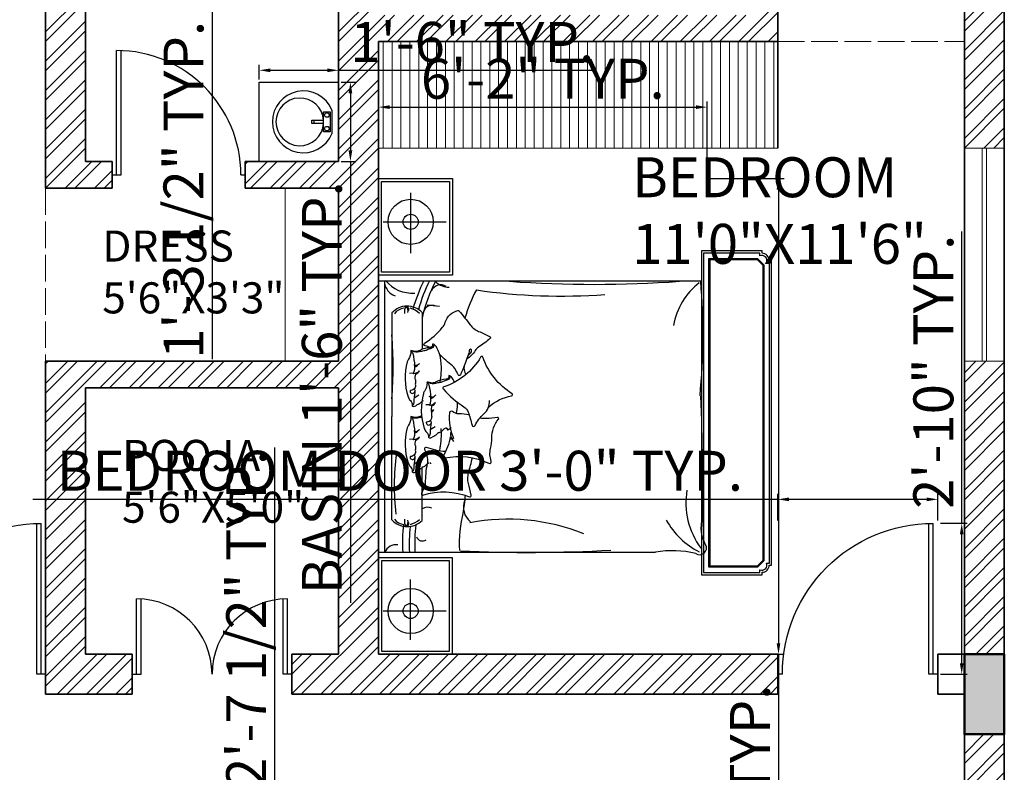
# Model space of a CAD drawing. Units: inches. Extents: x 4153 to 5577, y 785 to 1503.
# Tile 4 of 11: x 4480 to 4702, y 1217 to 1386. Entities that reach past the tile are written whole.
import ezdxf

# ---------------------------------------------------------------- set-up
doc = ezdxf.new("R2010")
doc.units = ezdxf.units.IN
doc.linetypes.add('ACAD_ISO02W100', pattern=[15, 12, -3])
for name, color, linetype, lineweight in [('A-ANNO-DIMS', 2, 'Continuous', 18), ('A-AREA-IDEN', 7, 'Continuous', 25), ('A-COLS', 7, 'Continuous', 50), ('A-DOOR', 3, 'Continuous', 25), ('A-FLOR-CASE', 32, 'Continuous', 18), ('A-FURN', 8, 'Continuous', 18), ('A-GLAZ', 4, 'Continuous', 18), ('A-WALL', 7, 'Continuous', 35), ('A-WALL-OVHD', 7, 'ACAD_ISO02W100', 18), ('Сантехника', 7, 'Continuous', 18)]:
    doc.layers.add(name, color=color, linetype=linetype, lineweight=lineweight)
doc.layers.add('A-FLOR-CASE-PATT', color=32, linetype='Continuous', lineweight=13, true_color=0xcd6928)
doc.layers.add('A-WALL-PATT', color=251, linetype='Continuous', lineweight=13, true_color=0x636466)
for name, color, linetype in [('FUR', 42, 'Continuous'), ('HA-FUR', 8, 'Continuous'), ('HA-P', 8, 'Continuous'), ('SAN', 5, 'Continuous'), ('SANTEH', 7, 'Continuous'), ('wood', 26, 'Continuous')]:
    doc.layers.add(name, color=color, linetype=linetype)
doc.styles.get("Standard").update_dxf_attribs({"font": 'arial.ttf'})
doc.dimstyles.new('ISO-25', dxfattribs={"dimtxt": 9, "dimasz": 2.5, "dimexe": 1.25, "dimexo": 0.625, "dimtad": 1, "dimlunit": 3, "dimtxsty": 'Standard', "dimcen": 2.5, "dimadec": 0, "dimazin": 0, "dimtfac": 1, "dimtmove": 0, "dimatfit": 3, "dimfxl": 1, "dimarcsym": 0})

# ---------------------------------------------------------------- blocks, each defined once
blk = doc.blocks.new('D1')
for p, q in [((1, 0), (1, 34)), ((2, 0), (2, 33.99)), ((0, 0), (2, 0)), ((35, 0), (36, 0))]:
    blk.add_line(p, q)
at = {"ltscale": 0.5}
blk.add_arc((1, 0), 34, 0, 90, dxfattribs=at)
blk = doc.blocks.new('D2')
for p, q in [((1, 0), (1, 28)), ((2, 0), (2, 27.98)), ((0, 0), (2, 0)), ((29, 0), (30, 0))]:
    blk.add_line(p, q)
at = {"ltscale": 0.5}
blk.add_arc((1, 0), 28, 0, 90, dxfattribs=at)
blk = doc.blocks.new('D3')
for p, q in [((1, 0), (1, 17)), ((2, 0), (2, 16.97)), ((34, 0), (34, 16.97)), ((35, 0), (35, 17)), ((0, 0), (2, 0)), ((36, 0), (34, 0))]:
    blk.add_line(p, q)
at = {"ltscale": 0.5}
for centre, start, end in [((1, 0), 0, 90), ((35, 0), 90, 180)]:
    blk.add_arc(centre, 17, start, end, dxfattribs=at)
blk = doc.blocks.new('A$C0A42580C')
at = {"layer": 'SAN'}
for p, q in [((0.2873, 0.0301), (0.2873, 0.4484)), ((2.8678, 0.0301), (2.8678, 0.4484)), ((0.0949, 0.2135), (0.4958, 0.2135)), ((3.0601, 0.2135), (2.6592, 0.2135))]:
    blk.add_line(p, q, dxfattribs=at)
for centre, radius in [((0.2873, 0.2135), 0.15), ((2.8678, 0.2135), 0.15), ((0.2873, 0.2135), 0.05), ((2.8678, 0.2135), 0.05)]:
    blk.add_circle(centre, radius, dxfattribs=at)
at = {"layer": 'wood'}
for p, q in [((0.6775, 0.8851), (0.6775, 2.1392)), ((2.4775, 0.8016), (2.4775, 1.838)), ((2.4775, 0), (2.4775, 0.8016)), ((1.5, 0.3423), (1.5016, 0.3142)), ((1.6633, 0.3438), (1.6434, 0.3761)), ((0.888, 0.289), (1.1327, 0.289)), ((1.4538, 0.2362), (1.434, 0.2685)), ((1.8919, 0.2362), (1.8721, 0.2685)), ((2.267, 0.289), (1.9163, 0.289)), ((1.2906, 0.2348), (1.2921, 0.2067)), ((1.7287, 0.2348), (1.7302, 0.2067)), ((0.8909, 0.089), (1.5775, 0.089)), ((2.2642, 0.089), (1.5775, 0.089)), ((0.6775, 0.039), (2.4775, 0.039)), ((0.6775, 0), (2.4775, 0))]:
    blk.add_line(p, q, dxfattribs=at)
blk.add_lwpolyline([(0.6775, 0), (0.6775, 0.8851)], dxfattribs=at)
for points in [[(1.516, 0.7294, -0.128392), (1.4401, 0.8834, 0.70791), (1.427, 0.8863, -0.16964), (1.1848, 0.6919, 0.664036), (1.184, 0.6776, -0.184649), (1.3819, 0.4332, 0.662242), (1.3969, 0.4309, 0.078539), (1.5137, 0.5669, -0.1736), (1.5484, 0.5947, -0.02159), (1.6357, 0.6205, 0.697276), (1.6379, 0.6405, -0.093019), (1.5606, 0.699, 0.216632), (1.4719, 0.7371, -2.511293)], [(1.6795, 0.4818, 0.263265), (1.7191, 0.4839, -0.026108), (1.743, 0.4973, 0.027613), (1.7137, 0.4764, -0.089259), (1.8403, 0.429, 0.662242), (1.8528, 0.4376, -0.162037), (1.8882, 0.732, 0.676499), (1.8733, 0.748, -0.160513), (1.7901, 0.7439, 0.07473), (1.7202, 0.7523, -0.187721), (1.5966, 0.7963, 0.70791), (1.5851, 0.7895, -0.010003), (1.5921, 0.7143, -0.07079), (1.5891, 0.6719, 0.099539)], [(1.1211, 0.3454, 0.032543), (1.1095, 0.3091, -0.658965), (1.0917, 0.3063, 0.074753), (0.9887, 0.4234, 0.100988), (0.953, 0.4429, -0.270711), (0.8753, 0.5273, -0.276825), (0.8775, 0.5337, -0.014937), (0.9701, 0.6081, 0.134834), (1.0135, 0.6643, -0.023706), (1.0474, 0.7372, -0.664036), (1.0616, 0.7394, -0.035987), (1.119, 0.6627, 0.118631), (1.1415, 0.6412, -0.132738), (1.1955, 0.5864)], [(1.1759, 0.5928, 0.013884), (1.1549, 0.6131, 0.174178), (1.1437, 0.6177, 0.104076), (1.1358, 0.6165, 0.389829), (1.1324, 0.6097, 0.296089), (1.1415, 0.6019, -0.036701), (1.1572, 0.5985, -0.040547), (1.3022, 0.543, -0.70791), (1.3021, 0.5296, -0.016811), (1.2631, 0.5085, 0.11866), (1.2414, 0.4904, -0.048791), (1.1649, 0.4055, 0.103757)], [(1.5674, 0.601, 0.057807), (1.5606, 0.5339, -0.173425), (1.5457, 0.49, 0.589988), (1.5538, 0.4706, 0.137312), (1.7236, 0.4985, 0.137312)], [(1.8113, 0.4446, -0.069098), (1.7831, 0.3187, 0.658965), (1.7961, 0.3062, -0.049789), (1.8516, 0.3234, -0.103757), (1.8905, 0.3233, 0.055725), (2.0203, 0.3103, -0.11866), (2.0478, 0.304, 0.016811), (2.0881, 0.2856, 0.70791), (2.0989, 0.2936, -0.16964), (2.1104, 0.604, 0.664036), (2.1001, 0.6139, 0.023706), (2.0214, 0.597, -0.134834), (1.9505, 0.5976, 0.012748), (1.8522, 0.6228)], [(1.3107, 0.4764, 0.145733), (1.3069, 0.4677, 0.488583), (1.3089, 0.4657, -0.012138), (1.3131, 0.4661, -0.125673), (1.3213, 0.4646, -0.750706)], [(1.3153, 0.4751, -0.274893), (1.3379, 0.4529, 0.051436), (1.3468, 0.4293, -0.086628), (1.3532, 0.4078, 0.040196), (1.3593, 0.3772, -0.184744), (1.3556, 0.3344, -2.554464)], [(1.317, 0.4683, -0.060098), (1.3283, 0.4571, -0.16247), (1.3313, 0.4487, 0.120018), (1.3493, 0.3815, -0.060072), (1.3541, 0.3695, -0.13107), (1.3541, 0.3395, -0.024415), (1.3534, 0.3373, 0.070398), (1.3503, 0.3233, 0.528689), (1.3524, 0.3216, -0.069388), (1.3557, 0.3222, -0.158233), (1.4075, 0.3065, 0.085461), (1.4255, 0.2981, 0.147196), (1.6571, 0.3041, 0.10985), (1.6823, 0.3191, -0.179095), (1.7126, 0.3319, -2.318897)], [(1.1013, 0.3688, 0.145733), (1.0975, 0.3601, 0.488583), (1.0995, 0.3581, -0.012138), (1.1036, 0.3585, -0.125673), (1.1119, 0.357, -0.750706)], [(1.1059, 0.3675, -0.274893), (1.1285, 0.3453, 0.051436), (1.1373, 0.3217, -0.086628), (1.1438, 0.3003, 0.040196), (1.1499, 0.2696, -0.184744), (1.1462, 0.2269, -2.554464)], [(1.1076, 0.3607, -0.060098), (1.1189, 0.3495, -0.16247), (1.1219, 0.3411, 0.120018), (1.1399, 0.2739, -0.060072), (1.1447, 0.2619, -0.13107), (1.1447, 0.2319, -0.024415), (1.144, 0.2297, 0.070398), (1.1409, 0.2157, 0.528689), (1.143, 0.2141, -0.069388), (1.1463, 0.2146, -0.158233), (1.1981, 0.1989, 0.085461), (1.2161, 0.1905, 0.147196), (1.4477, 0.1965, 0.10985), (1.4728, 0.2115, -0.179095), (1.5032, 0.2244, -2.318897)], [(1.3509, 0.3219, -0.117141), (1.3688, 0.335, -0.025084), (1.4533, 0.348, 0.033691)], [(1.4359, 0.3803, -0.198519), (1.452, 0.3494, 0.826402), (1.4558, 0.349, 0.095956), (1.4561, 0.3528, 0.242899), (1.4461, 0.3686, -17.523452)], [(1.5447, 0.3525, -0.083557), (1.507, 0.3546, 0.203162), (1.4851, 0.3792, -0.208037), (1.5043, 0.3409, 0.124669), (1.4432, 0.3469, 0.965934)], [(1.5394, 0.3688, 0.145733), (1.5356, 0.3601, 0.488583), (1.5376, 0.3581, -0.012138), (1.5418, 0.3585, -0.125673), (1.55, 0.357, -0.750706)], [(1.5447, 0.3525, -0.008229), (1.5728, 0.3519, 0.033691)], [(1.5728, 0.3519, -0.46905), (1.6152, 0.321, 0.420988), (1.62, 0.3169, 0.857652), (1.6221, 0.3484, 0.548526)], [(1.603, 0.3451, -0.099719), (1.6221, 0.3484, 0.102691)], [(1.6214, 0.3487, -0.010168), (1.6558, 0.3447, 0.033691), (1.6907, 0.3423, -0.220869), (1.7148, 0.3311, -0.288972)], [(1.2265, 0.2728, -0.198519), (1.2426, 0.2418, 0.826402), (1.2463, 0.2415, 0.095956), (1.2467, 0.2452, 0.242899), (1.2366, 0.2611, -17.523452)], [(1.3353, 0.2449, -0.083557), (1.2976, 0.247, 0.203162), (1.2757, 0.2717, -0.208037), (1.2948, 0.2333, 0.124669), (1.2338, 0.2393, 0.965934)], [(1.5721, 0.286, 0.022869), (1.578, 0.2739, -0.060072), (1.5828, 0.2619, -0.13107), (1.5828, 0.2319, -0.024415), (1.5821, 0.2297, 0.070398), (1.579, 0.2157, 0.528689), (1.5811, 0.2141, -0.069388), (1.5844, 0.2146, -0.158233), (1.6362, 0.1989, 0.085461), (1.6542, 0.1905, 0.147196), (1.8858, 0.1965, 0.10985), (1.911, 0.2115, -0.179095), (1.9413, 0.2244, -2.318897)], [(1.5838, 0.2873, 0.023398), (1.588, 0.2696, -0.184744), (1.5843, 0.2269, -2.554464)], [(1.6646, 0.2728, -0.198519), (1.6807, 0.2418, 0.826402), (1.6845, 0.2415, 0.095956), (1.6848, 0.2452, 0.242899), (1.6748, 0.2611, -17.523452)], [(1.7734, 0.2449, -0.083557), (1.7357, 0.247, 0.203162), (1.7138, 0.2717, -0.208037), (1.733, 0.2333, 0.124669), (1.6719, 0.2393, 0.965934)], [(1.1415, 0.2143, -0.117141), (1.1594, 0.2274, -0.025084), (1.2439, 0.2405, 0.033691)], [(1.3353, 0.2449, -0.008229), (1.3633, 0.2443, 0.033691)], [(1.3633, 0.2443, -0.46905), (1.4058, 0.2134, 0.420988), (1.4106, 0.2093, 0.857652), (1.4127, 0.2408, 0.548526)], [(1.3936, 0.2375, -0.099719), (1.4127, 0.2408, 0.102691)], [(1.412, 0.2411, -0.010168), (1.4464, 0.2371, 0.033691), (1.4812, 0.2348, -0.220869), (1.5054, 0.2235, -0.288972)], [(1.5796, 0.2143, -0.117141), (1.5975, 0.2274, -0.025084), (1.682, 0.2405, 0.033691)], [(1.7734, 0.2449, -0.008229), (1.8015, 0.2443, 0.033691)], [(1.8015, 0.2443, -0.46905), (1.8439, 0.2134, 0.420988), (1.8487, 0.2093, 0.857652), (1.8508, 0.2408, 0.548526)], [(1.8317, 0.2375, -0.099719), (1.8508, 0.2408, 0.102691)], [(1.8501, 0.2411, -0.010168), (1.8845, 0.2371, 0.033691), (1.9193, 0.2348, -0.220869), (1.9435, 0.2235, -0.288972)]]:
    blk.add_lwpolyline(points, format="xyb", dxfattribs=at)
for points in [[(0.64, 0), (0, 0), (0, 0.49), (0.64, 0.49)], [(0.62, 0.02), (0.02, 0.02), (0.02, 0.47), (0.62, 0.47)], [(2.515, 0), (3.155, 0), (3.155, 0.49), (2.515, 0.49)], [(2.535, 0.02), (3.135, 0.02), (3.135, 0.47), (2.535, 0.47)]]:
    blk.add_lwpolyline(points, close=True, dxfattribs=at)
for centre, radius, start, end in [((2.3125, 2.3833), 0.2443, 254.1515, 300.95574), ((2.4501, 2.1309), 0.0445, 324.18954, 118.92203), ((1.0344, -2.14), 4.292, 84.56078, 94.7164), ((1.0494, 2.4026), 0.4515, 217.47941, 260.35986), ((2.0208, -11.0786), 13.2288, 88.75549, 92.51133), ((2.1491, 2.5471), 0.5083, 260.65485, 306.44155), ((2.0168, 2.3573), 0.5127, 299.08175, 333.44367), ((3.1371, 1.9502), 0.669, 166.6404, 189.65708), ((-7.0839, 1.4328), 7.7858, 355.84817, 4.15183), ((-3.167, 1.2143), 3.9465, 351.77286, 4.18386), ((-7.2439, 0.9937), 9.7233, 357.34474, 3.23068), ((3.5803, 0.8622), 1.3213, 157.81295, 191.15154), ((1.1611, 1.4181), 0.8768, 241.21362, 254.41879), ((2.181, 0.6859), 0.1221, 247.37754, 321.13165), ((1.2583, 0.6364), 0.0695, 238.58923, 301.92671), ((1.4714, 0.0722), 0.4528, 80.62397, 88.74059), ((1.7861, -2.1601), 2.7557, 80.89877, 83.46656), ((2.4192, 1.3819), 0.8461, 255.77539, 273.25587), ((0.5904, 0.4689), 0.13, 317.38218, 359.70393), ((1.3546, 0.4469), 0.0529, 114.21284, 146.15395), ((2.6126, -2.3504), 3.1201, 113.83178, 114.21284), ((1.4035, -0.3388), 0.8693, 79.71489, 80.62397), ((1.6301, 0.4539), 0.0342, 31.14095, 54.95422), ((1.6709, 0.4489), 0.0156, 131.9623, 212.08127), ((1.5664, 0.4154), 0.1086, 24.20989, 31.14095), ((1.6627, 0.4587), 0.00309, 275.52245, 24.20989), ((0.7723, 0.4131), 0.0674, 147.68233, 245.79865), ((0.0312, 0.4583), 0.8174, 350.42368, 356.2506), ((2.4032, -2.458), 3.1201, 113.55686, 114.21284), ((1.2046, 0.2912), 0.121, 99.42032, 113.55686), ((1.2774, -0.1478), 0.5659, 95.90379, 99.42032), ((1.2626, -0.005), 0.4223, 88.74059, 95.90379), ((1.2619, -0.0354), 0.4528, 80.62397, 88.74059), ((1.1941, -0.4464), 0.8693, 79.45871, 80.62397), ((1.6729, 0.4422), 0.0178, 140.41793, 157.63267), ((1.7007, -0.005), 0.4223, 88.74059, 95.90379), ((1.7235, 0.4818), 0.0777, 212.08127, 227.364), ((1.6635, 0.4499), 0.00568, 95.52245, 140.41793), ((1.6391, 0.3902), 0.0469, 17.32618, 47.364), ((1.7106, 0.4125), 0.028, 197.32618, 226.17302), ((1.6431, 0.3422), 0.0695, 26.61764, 46.17302), ((1.7001, -0.0354), 0.4528, 80.62397, 88.74059), ((1.6322, -0.4464), 0.8693, 78.43923, 80.62397), ((1.1611, 1.3191), 1.0568, 242.76671, 257.10398), ((1.1611, 1.3191), 1.0937, 243.75553, 254.4906), ((0.9021, 0.3562), 0.0605, 155.8342, 254.41058), ((1.1452, 0.3394), 0.0529, 114.21284, 146.15395), ((1.4207, 0.3463), 0.0342, 31.14095, 54.95422), ((1.4614, 0.3413), 0.0156, 131.9623, 212.08127), ((1.4635, 0.3347), 0.0178, 140.41793, 157.63267), ((1.4541, 0.3424), 0.00568, 95.52245, 140.41793), ((1.357, 0.3078), 0.1086, 24.20989, 31.14095), ((1.4533, 0.3511), 0.00309, 275.52245, 24.20989), ((1.8202, 0.431), 0.1287, 206.61764, 215.96192), ((1.715, 0.3349), 0.00379, 207.1817, 328.02977), ((1.6975, 0.3419), 0.023, 350.76434, 35.96192), ((1.7058, 0.3406), 0.0145, 328.02977, 350.76434), ((1.9016, 0.3347), 0.0178, 140.41793, 157.63267), ((1.9522, 0.3743), 0.0777, 212.08127, 227.364), ((1.8922, 0.3424), 0.00568, 95.52245, 140.41793), ((2.2511, 0.3256), 0.071, 155.86842, 211.04513), ((1.1611, 1.2816), 1.0937, 243.75553, 254.38927), ((0.9846, 0.1903), 0.1381, 134.39284, 227.23745), ((0.9986, 0.1735), 0.1427, 136.58239, 164.9725), ((1.5012, 0.305), 0.028, 197.32618, 226.17302), ((1.4337, 0.2347), 0.0695, 26.61764, 46.17302), ((1.6108, 0.3235), 0.1287, 206.61764, 215.96192), ((1.8678, 0.2827), 0.0469, 17.32618, 47.364), ((1.9393, 0.305), 0.028, 197.32618, 226.17302), ((1.8718, 0.2347), 0.0695, 26.61764, 46.17302), ((2.0489, 0.3235), 0.1287, 206.61764, 215.96192), ((2.1565, 0.1735), 0.1427, 15.0275, 43.41761), ((2.1704, 0.1903), 0.1381, 312.76255, 45.60716), ((2.3616, 0.2915), 0.0419, 290.78583, 35.36309), ((0.5293, 0.2241), 0.2307, 309.63048, 4.27465), ((0.8802, 0.1371), 0.0592, 81.47786, 123.11925), ((0.8698, 0.1793), 0.0229, 77.14902, 159.1786), ((1.5055, 0.2273), 0.00379, 207.1817, 328.02977), ((1.4881, 0.2344), 0.023, 350.76434, 35.96192), ((1.4964, 0.233), 0.0145, 328.02977, 350.76434), ((1.9436, 0.2273), 0.00379, 207.1817, 328.02977), ((1.9262, 0.2344), 0.023, 350.76434, 35.96192), ((1.9345, 0.233), 0.0145, 328.02977, 350.76434), ((2.2749, 0.1371), 0.0592, 56.88075, 98.52214), ((2.2853, 0.1793), 0.0229, 20.8214, 102.85098), ((2.4192, 1.2667), 1.0261, 263.09035, 273.25587), ((2.4192, 1.2667), 1.0629, 263.94374, 273.25587), ((0.8396, 0.185), 0.0112, 314.89662, 45.10338), ((0.8413, 0.1846), 0.0128, 299.47062, 57.44416), ((0.8844, 0.2286), 0.0569, 229.70587, 281.11527), ((0.9466, 0.1765), 0.0862, 185.53723, 234.68694), ((2.2085, 0.1765), 0.0862, 305.31306, 354.46277), ((2.2706, 0.2286), 0.0569, 258.88473, 310.29413), ((2.4192, 1.2218), 1.0629, 263.23622, 273.25587), ((2.3138, 0.1846), 0.0128, 122.55584, 240.52938), ((2.3154, 0.185), 0.0112, 134.89662, 225.10338), ((0.6729, 0.151), 0.1135, 279.23824, 338.73819), ((1.2481, -2.5919), 2.6893, 85.4722, 94.5278), ((2.0447, 1.7022), 1.5979, 262.13639, 276.48786), ((2.508, 0.1152), 0.0792, 169.94668, 248.24015)]:
    blk.add_arc(centre, radius, start, end, dxfattribs=at)
blk = doc.blocks.new('A$C623F1DA0')
at = {"layer": 'FUR'}
blk.add_lwpolyline([(0.628, 2.912, 0.414214), (0.562, 2.978), (0.562, 3), (0, 3), (0, 0), (0.562, 0), (0.562, 0.022, 0.414214), (0.628, 0.088), (0.65, 0.088), (0.65, 2.912)], format="xyb", close=True, dxfattribs=at)
at = {"layer": 'HA-FUR'}
blk.add_lwpolyline([(0.6034, 2.892, 0.710288), (0.542, 2.9534), (0.542, 2.98), (0.02, 2.98), (0.02, 0.02), (0.542, 0.02), (0.542, 0.0466, 0.710288), (0.6034, 0.108), (0.63, 0.108), (0.63, 2.892)], format="xyb", close=True, dxfattribs=at)
at = {"layer": 'HA-P'}
for points in [[(0.07, 2.93), (0.5213, 2.93), (0.58, 2.8713), (0.58, 0.1287), (0.5213, 0.07), (0.07, 0.07)], [(0.08, 2.92), (0.5171, 2.92), (0.57, 2.8671), (0.57, 0.1329), (0.5171, 0.08), (0.08, 0.08)]]:
    blk.add_lwpolyline(points, close=True, dxfattribs=at)
blk = doc.blocks.new('r11')
at = {"layer": 'SANTEH', "ltscale": 5}
for p, q in [((0, 0), (600, 0)), ((0, -600), (0, 0)), ((600, 0), (600, -600)), ((210.5, -50), (389.5, -50)), ((210.5, -50), (210.5, -50)), ((223.8, -63.2), (376.2, -63.2)), ((223.8, -113.2), (223.8, -63.2)), ((232.7, -78.7), (249.2, -69.1)), ((249.2, -69.1), (265.7, -78.7)), ((334.3, -78.7), (350.8, -69.1)), ((350.8, -69.1), (367.3, -78.7)), ((376.2, -63.2), (376.2, -113.2)), ((376.2, -113.2), (223.8, -113.2)), ((232.7, -97.7), (232.7, -78.7)), ((249.2, -107.2), (232.7, -97.7)), ((265.7, -97.7), (249.2, -107.2)), ((265.7, -78.7), (265.7, -97.7)), ((288, -201.6), (288, -113.2)), ((312, -113.2), (312, -201.6)), ((334.3, -97.7), (334.3, -78.7)), ((350.8, -107.2), (334.3, -97.7)), ((367.3, -97.7), (350.8, -107.2)), ((367.3, -78.7), (367.3, -97.7)), ((312, -184.3), (288, -184.3)), ((312, -201.6), (288, -201.6)), ((600, -600), (0, -600))]:
    blk.add_line(p, q, dxfattribs=at)
for centre, radius, start, end in [((300, -266.2), 234, 112.50001, 67.49999), ((300, -293), 180.2, 93.8183, 86.1817)]:
    blk.add_arc(centre, radius, start, end, dxfattribs=at)
blk = doc.blocks.new('WINDOW-48IN')
for p, q in [((0, 9), (0, 0)), ((48, 9), (48, 0)), ((0, 5), (48, 5)), ((0, 4), (48, 4))]:
    blk.add_line(p, q)
blk = doc.blocks.new('COL-9X18IN')
at = {"transparency": 33554687}
h = blk.add_hatch(color=256, dxfattribs=at)
h.dxf.hatch_style = 1
h.paths.add_polyline_path([(9, 18), (0, 18), (0, 0), (9, 0)])
blk.add_lwpolyline([(0, 18), (9, 18), (9, 0), (0, 0)], close=True)
blk = doc.blocks.new('*D112')
at = {"layer": 'A-ANNO-DIMS', "color": 0, "lineweight": -2, "transparency": 16777216}
for p, q in [((4635.6, 1350.66), (4652.3, 1350.66)), ((4651.05, 1348.16), (4651.05, 1245.99)), ((4635.6, 1243.49), (4652.3, 1243.49)), ((4651.05, 1243.49), (4651.05, 1099.34))]:
    blk.add_line(p, q, dxfattribs=at)
at = {"layer": 'A-ANNO-DIMS', "color": 0, "transparency": 16777216}
for points in [[(4650.63, 1348.16), (4651.47, 1348.16), (4651.05, 1350.66)], [(4650.63, 1245.99), (4651.47, 1245.99), (4651.05, 1243.49)]]:
    blk.add_solid(points, dxfattribs=at)
at = {"layer": 'Defpoints', "color": 0, "transparency": 16777216}
for p in [(4634.98, 1350.66), (4634.98, 1243.49), (4651.05, 1243.49)]:
    blk.add_point(p, dxfattribs=at)
at = {"layer": 'A-ANNO-DIMS', "color": 0, "transparency": 16777216, "insert": (4645.77, 1170.17), "char_height": 9, "attachment_point": 5, "rotation": 90}
blk.add_mtext('BED GROUP 8\'-11" TYP.', dxfattribs=at)
blk = doc.blocks.new('*D113')
at = {"layer": 'A-ANNO-DIMS', "color": 0, "lineweight": -2, "transparency": 16777216}
for p, q in [((4560.93, 1351.29), (4560.93, 1367.99)), ((4563.43, 1366.74), (4632.48, 1366.74)), ((4634.98, 1351.29), (4634.98, 1367.99))]:
    blk.add_line(p, q, dxfattribs=at)
at = {"layer": 'A-ANNO-DIMS', "color": 0, "transparency": 16777216}
for points in [[(4563.43, 1367.15), (4563.43, 1366.32), (4560.93, 1366.74)], [(4632.48, 1367.15), (4632.48, 1366.32), (4634.98, 1366.74)]]:
    blk.add_solid(points, dxfattribs=at)
at = {"layer": 'Defpoints', "color": 0, "transparency": 16777216}
for p in [(4634.98, 1366.74), (4560.93, 1350.66), (4634.98, 1350.66)]:
    blk.add_point(p, dxfattribs=at)
at = {"layer": 'A-ANNO-DIMS', "color": 0, "transparency": 16777216, "insert": (4597.95, 1371.96), "char_height": 9, "attachment_point": 5}
blk.add_mtext('6\'-2" TYP.', dxfattribs=at)
blk = doc.blocks.new('*D119')
at = {"layer": 'A-ANNO-DIMS', "color": 0, "lineweight": -2, "transparency": 16777216}
for p, q in [((4520.35, 1404.11), (4524.69, 1404.11)), ((4523.44, 1401.61), (4523.44, 1391.22)), ((4520.35, 1388.72), (4524.69, 1388.72)), ((4523.44, 1388.72), (4523.44, 1309.99))]:
    blk.add_line(p, q, dxfattribs=at)
at = {"layer": 'A-ANNO-DIMS', "color": 0, "transparency": 16777216}
for points in [[(4523.02, 1401.61), (4523.86, 1401.61), (4523.44, 1404.11)], [(4523.02, 1391.22), (4523.86, 1391.22), (4523.44, 1388.72)]]:
    blk.add_solid(points, dxfattribs=at)
at = {"layer": 'Defpoints', "color": 0, "transparency": 16777216}
for p in [(4519.72, 1404.11), (4519.72, 1388.72), (4523.44, 1388.72)]:
    blk.add_point(p, dxfattribs=at)
at = {"layer": 'A-ANNO-DIMS', "color": 0, "transparency": 16777216, "insert": (4518.16, 1348.1), "char_height": 9, "attachment_point": 5, "rotation": 90}
blk.add_mtext('1\'-3 1/2" TYP.', dxfattribs=at)
blk = doc.blocks.new('*D120')
at = {"layer": 'A-ANNO-DIMS', "color": 0, "lineweight": -2, "transparency": 16777216}
for p, q in [((4552.55, 1372.36), (4555.86, 1372.36)), ((4554.61, 1369.86), (4554.61, 1356.99)), ((4552.55, 1354.49), (4555.86, 1354.49)), ((4554.61, 1354.49), (4554.61, 1255.05))]:
    blk.add_line(p, q, dxfattribs=at)
at = {"layer": 'A-ANNO-DIMS', "color": 0, "transparency": 16777216}
for points in [[(4554.19, 1369.86), (4555.02, 1369.86), (4554.61, 1372.36)], [(4554.19, 1356.99), (4555.02, 1356.99), (4554.61, 1354.49)]]:
    blk.add_solid(points, dxfattribs=at)
at = {"layer": 'Defpoints', "color": 0, "transparency": 16777216}
for p in [(4551.93, 1372.36), (4551.93, 1354.49), (4554.61, 1354.49)]:
    blk.add_point(p, dxfattribs=at)
at = {"layer": 'A-ANNO-DIMS', "color": 0, "transparency": 16777216, "insert": (4549.33, 1303.52), "char_height": 9, "attachment_point": 5, "rotation": 90}
blk.add_mtext('BASIN 1\'-6" TYP.', dxfattribs=at)
blk = doc.blocks.new('*D121')
at = {"layer": 'A-ANNO-DIMS', "color": 0, "lineweight": -2, "transparency": 16777216}
for p, q in [((4534.06, 1372.98), (4534.06, 1376.29)), ((4551.93, 1372.98), (4551.93, 1376.29)), ((4536.56, 1375.04), (4549.43, 1375.04)), ((4551.93, 1375.04), (4609.69, 1375.04))]:
    blk.add_line(p, q, dxfattribs=at)
at = {"layer": 'A-ANNO-DIMS', "color": 0, "transparency": 16777216}
for points in [[(4536.56, 1375.45), (4536.56, 1374.62), (4534.06, 1375.04)], [(4549.43, 1375.45), (4549.43, 1374.62), (4551.93, 1375.04)]]:
    blk.add_solid(points, dxfattribs=at)
at = {"layer": 'Defpoints', "color": 0, "transparency": 16777216}
for p in [(4551.93, 1375.04), (4534.06, 1372.36), (4551.93, 1372.36)]:
    blk.add_point(p, dxfattribs=at)
at = {"layer": 'A-ANNO-DIMS', "color": 0, "transparency": 16777216, "insert": (4582.06, 1380.26), "char_height": 9, "attachment_point": 5}
blk.add_mtext('1\'-6" TYP.', dxfattribs=at)
blk = doc.blocks.new('*D129')
at = {"layer": 'A-ANNO-DIMS', "color": 0, "lineweight": -2, "transparency": 16777216}
for p, q in [((4537.57, 1210.35), (4537.57, 1290.09)), ((4542.33, 1210.35), (4536.32, 1210.35)), ((4537.57, 1181.43), (4537.57, 1207.85)), ((4542.33, 1178.93), (4536.32, 1178.93))]:
    blk.add_line(p, q, dxfattribs=at)
at = {"layer": 'A-ANNO-DIMS', "color": 0, "transparency": 16777216}
for points in [[(4537.15, 1207.85), (4537.99, 1207.85), (4537.57, 1210.35)], [(4537.15, 1181.43), (4537.99, 1181.43), (4537.57, 1178.93)]]:
    blk.add_solid(points, dxfattribs=at)
at = {"layer": 'Defpoints', "color": 0, "transparency": 16777216}
for p in [(4537.57, 1210.35), (4542.96, 1210.35), (4542.96, 1178.93)]:
    blk.add_point(p, dxfattribs=at)
at = {"layer": 'A-ANNO-DIMS', "color": 0, "transparency": 16777216, "insert": (4532.29, 1251.47), "char_height": 9, "attachment_point": 5, "rotation": 90}
blk.add_mtext('2\'-7 1/2" TYP.', dxfattribs=at)
blk = doc.blocks.new('*D142')
at = {"layer": 'A-ANNO-DIMS', "color": 0, "lineweight": -2, "transparency": 16777216}
for p, q in [((4650.93, 1278.39), (4483.05, 1278.39)), ((4650.93, 1273.61), (4650.93, 1279.64)), ((4684.43, 1278.39), (4653.43, 1278.39)), ((4686.93, 1273.61), (4686.93, 1279.64))]:
    blk.add_line(p, q, dxfattribs=at)
at = {"layer": 'A-ANNO-DIMS', "color": 0, "transparency": 16777216}
for points in [[(4653.43, 1278.81), (4653.43, 1277.97), (4650.93, 1278.39)], [(4684.43, 1278.81), (4684.43, 1277.97), (4686.93, 1278.39)]]:
    blk.add_solid(points, dxfattribs=at)
at = {"layer": 'Defpoints', "color": 0, "transparency": 16777216}
for p in [(4650.93, 1278.39), (4650.93, 1272.99), (4686.93, 1272.99)]:
    blk.add_point(p, dxfattribs=at)
at = {"layer": 'A-ANNO-DIMS', "color": 0, "transparency": 16777216, "insert": (4565.74, 1283.67), "char_height": 9, "attachment_point": 5}
blk.add_mtext('BEDROOM DOOR 3\'-0" TYP.', dxfattribs=at)
blk = doc.blocks.new('*D143')
at = {"layer": 'A-ANNO-DIMS', "color": 0, "lineweight": -2, "transparency": 16777216}
for p, q in [((4692.33, 1272.99), (4692.33, 1338.74)), ((4687.55, 1272.99), (4693.58, 1272.99)), ((4692.33, 1241.49), (4692.33, 1270.49)), ((4687.55, 1238.99), (4693.58, 1238.99))]:
    blk.add_line(p, q, dxfattribs=at)
at = {"layer": 'A-ANNO-DIMS', "color": 0, "transparency": 16777216}
for points in [[(4691.91, 1270.49), (4692.74, 1270.49), (4692.33, 1272.99)], [(4691.91, 1241.49), (4692.74, 1241.49), (4692.33, 1238.99)]]:
    blk.add_solid(points, dxfattribs=at)
at = {"layer": 'Defpoints', "color": 0, "transparency": 16777216}
for p in [(4686.93, 1272.99), (4692.33, 1272.99), (4686.93, 1238.99)]:
    blk.add_point(p, dxfattribs=at)
at = {"layer": 'A-ANNO-DIMS', "color": 0, "transparency": 16777216, "insert": (4687.11, 1307.12), "char_height": 9, "attachment_point": 5, "rotation": 90}
blk.add_mtext('2\'-10" TYP.', dxfattribs=at)

msp = doc.modelspace()

# ---------------------------------------------------------------- hatches: boundary and pattern name
at = {"layer": 'A-FLOR-CASE-PATT'}
h = msp.add_hatch(dxfattribs=at)
h.set_pattern_fill('ANSI31', color=256, scale=0.6299213, angle=45, style=0)
h.paths.add_polyline_path([(4560.927, 1357.488), (4650.927, 1357.488), (4650.927, 1381.488), (4560.927, 1381.488)])
at = {"layer": 'A-WALL-PATT', "transparency": 33554687}
h = msp.add_hatch(dxfattribs=at)
h.set_pattern_fill('ANSI32', color=256, scale=0.49)
h.paths.add_polyline_path([(4344.927, 1138.488), (4281.927, 1138.488), (4281.927, 1234.488), (4296.927, 1234.488), (4296.927, 1243.488), (4269.927, 1243.488), (4269.927, 1234.488), (4275.927, 1234.488), (4275.927, 1138.488), (4203.927, 1138.488), (4203.927, 1168.488), (4194.927, 1168.488), (4194.927, 1088.988), (4203.927, 1088.988), (4203.927, 1129.488), (4338.927, 1129.488), (4338.927, 1105.488), (4344.927, 1105.488)])
h.paths.add_polyline_path([(4203.927, 1040.988), (4194.927, 1040.988), (4194.927, 1009.488), (4203.927, 1009.488)])
h.paths.add_polyline_path([(4278.927, 1000.488), (4203.927, 1000.488), (4203.927, 991.488), (4278.927, 991.488)])
h.paths.add_polyline_path([(4203.927, 991.488), (4194.927, 991.488), (4194.927, 910.488), (4203.927, 910.488)])
h.paths.add_polyline_path([(4335.927, 907.488), (4203.927, 907.488), (4203.927, 901.488), (4335.927, 901.488)])
h.paths.add_polyline_path([(4344.927, 1057.488), (4338.927, 1057.488), (4338.927, 1000.488), (4344.927, 1000.488)])
h.paths.add_polyline_path([(4335.927, 1000.488), (4326.927, 1000.488), (4326.927, 991.488), (4335.927, 991.488)])
h.paths.add_polyline_path([(4368.927, 1000.488), (4344.927, 1000.488), (4344.927, 991.488), (4368.927, 991.488)])
h.paths.add_polyline_path([(4440.927, 1000.488), (4416.927, 1000.488), (4416.927, 991.488), (4440.927, 991.488)])
h.paths.add_polyline_path([(4449.927, 1120.488), (4440.927, 1120.488), (4440.927, 1000.488), (4449.927, 1000.488)])
h.paths.add_polyline_path([(4473.927, 1000.488), (4458.927, 1000.488), (4458.927, 991.488), (4473.927, 991.488)])
h.paths.add_polyline_path([(4638.927, 1000.488), (4545.927, 1000.488), (4545.927, 991.488), (4638.927, 991.488)])
h.paths.add_polyline_path([(4701.927, 1036.488), (4692.927, 1036.488), (4692.927, 1009.488), (4701.927, 1009.488)])
h.paths.add_polyline_path([(4692.927, 1000.488), (4686.927, 1000.488), (4686.927, 991.488), (4692.927, 991.488)])
h.paths.add_polyline_path([(4701.927, 1132.488), (4692.927, 1132.488), (4692.927, 1108.488), (4701.927, 1108.488)])
h.paths.add_polyline_path([(4701.927, 1225.488), (4692.927, 1225.488), (4692.927, 1204.488), (4701.927, 1204.488)])
h.paths.add_polyline_path([(4650.927, 1243.488), (4560.927, 1243.488), (4560.927, 1265.228), (4560.927, 1381.488), (4650.927, 1381.488), (4650.927, 1393.488), (4644.927, 1393.488), (4644.927, 1387.488), (4560.927, 1387.488), (4560.927, 1435.488), (4551.927, 1435.488), (4551.927, 1354.488), (4530.927, 1354.488), (4530.927, 1348.488), (4551.927, 1348.488), (4551.927, 1309.488), (4485.927, 1309.488), (4485.927, 1234.488), (4505.427, 1234.488), (4505.427, 1243.488), (4494.927, 1243.488), (4494.927, 1303.488), (4551.927, 1303.488), (4551.927, 1243.488), (4541.427, 1243.488), (4541.427, 1234.488), (4650.927, 1234.488)])
h.paths.add_polyline_path([(4701.927, 1426.488), (4692.927, 1426.488), (4692.927, 1357.488), (4701.927, 1357.488)])
h.paths.add_polyline_path([(4701.927, 1309.488), (4692.927, 1309.488), (4692.927, 1243.488), (4701.927, 1243.488)])
h.paths.add_polyline_path([(4692.927, 1444.488), (4608.927, 1444.488), (4608.927, 1435.488), (4644.927, 1435.488), (4644.927, 1423.488), (4650.927, 1423.488), (4650.927, 1435.488), (4692.927, 1435.488)])
h.paths.add_polyline_path([(4497.927, 1444.488), (4479.927, 1444.488), (4479.927, 1435.488), (4485.927, 1435.488), (4485.927, 1348.488), (4500.927, 1348.488), (4500.927, 1354.488), (4494.927, 1354.488), (4494.927, 1435.488), (4497.927, 1435.488)])
h.paths.add_polyline_path([(4551.927, 1444.488), (4545.927, 1444.488), (4545.927, 1435.488), (4551.927, 1435.488)])
h.paths.add_polyline_path([(4572.927, 1444.488), (4569.927, 1444.488), (4569.927, 1435.488), (4572.927, 1435.488)])
h.paths.add_polyline_path([(4431.927, 1444.488), (4356.927, 1444.488), (4356.927, 1435.488), (4431.927, 1435.488)])
h.paths.add_polyline_path([(4284.927, 1444.488), (4203.927, 1444.488), (4203.927, 1435.488), (4284.927, 1435.488)])
h.paths.add_polyline_path([(4203.927, 1426.488), (4194.927, 1426.488), (4194.927, 1293.488), (4203.927, 1293.488), (4203.927, 1295.242)])
h.paths.add_polyline_path([(4347.927, 1435.488), (4338.927, 1435.488), (4338.927, 1243.488), (4332.927, 1243.488), (4332.927, 1234.488), (4431.927, 1234.488), (4431.927, 1243.488), (4347.927, 1243.488)])
h.paths.add_polyline_path([(4239.927, 1243.488), (4203.927, 1243.488), (4203.927, 1234.488), (4239.927, 1234.488)], flags=17)
h.paths.add_polyline_path([(4203.927, 1225.488), (4194.927, 1225.488), (4194.927, 1198.488), (4203.927, 1198.488)], flags=17)

# ---------------------------------------------------------------- linework, layer by layer
at = {"layer": 'A-FLOR-CASE'}
for p, q in [((4560.927, 1357.488), (4650.927, 1357.488)), ((4539.927, 1309.488), (4539.927, 1348.488))]:
    msp.add_line(p, q, dxfattribs=at)
at = {"layer": 'A-WALL'}
for p, q in [((4701.927, 1444.488), (4701.927, 901.488)), ((4485.927, 1348.488), (4485.927, 1435.488)), ((4494.927, 1354.488), (4494.927, 1435.488)), ((4551.927, 1354.488), (4551.927, 1435.488)), ((4692.927, 1435.488), (4692.927, 1243.488)), ((4650.927, 1357.488), (4650.927, 1393.488)), ((4560.927, 1243.488), (4560.927, 1381.488)), ((4560.927, 1381.488), (4650.927, 1381.488)), ((4494.927, 1354.488), (4500.927, 1354.488)), ((4500.927, 1348.488), (4500.927, 1354.488)), ((4530.927, 1354.488), (4551.927, 1354.488)), ((4530.927, 1348.488), (4530.927, 1354.488)), ((4485.927, 1348.488), (4500.927, 1348.488)), ((4530.927, 1348.488), (4551.927, 1348.488)), ((4551.927, 1309.488), (4551.927, 1348.488)), ((4485.927, 1234.488), (4485.927, 1309.488)), ((4485.927, 1309.488), (4551.927, 1309.488)), ((4494.927, 1243.488), (4494.927, 1303.488)), ((4494.927, 1303.488), (4551.927, 1303.488)), ((4551.927, 1243.488), (4551.927, 1303.488)), ((4494.927, 1243.488), (4505.427, 1243.488)), ((4505.427, 1243.488), (4505.427, 1234.488)), ((4541.427, 1243.488), (4541.427, 1234.488)), ((4541.427, 1243.488), (4551.927, 1243.488)), ((4560.927, 1243.488), (4650.927, 1243.488)), ((4650.927, 1243.488), (4650.927, 1234.488)), ((4686.927, 1243.488), (4686.927, 1234.488)), ((4686.927, 1243.488), (4692.927, 1243.488)), ((4485.927, 1234.488), (4505.427, 1234.488)), ((4541.427, 1234.488), (4650.927, 1234.488)), ((4686.927, 1234.488), (4692.927, 1234.488)), ((4692.927, 1234.488), (4692.927, 1000.488))]:
    msp.add_line(p, q, dxfattribs=at)
at = {"layer": 'A-WALL-OVHD', "ltscale": 0.5}
for p, q in [((4650.927, 1381.488), (4692.927, 1381.488)), ((4485.927, 1348.488), (4485.927, 1309.488))]:
    msp.add_line(p, q, dxfattribs=at)

# ---------------------------------------------------------------- block references
at = {"layer": 'A-COLS'}
msp.add_blockref('COL-9X18IN', (4692.927, 1225.488), dxfattribs=at)
at = {"layer": 'A-DOOR'}
for name, p in [('D2', (4500.927, 1351.488)), ('D3', (4505.427, 1238.988))]:
    msp.add_blockref(name, p, dxfattribs=at)
at = {"layer": 'A-DOOR', "xscale": -1}
for p in [(4485.927, 1238.988), (4686.927, 1238.988)]:
    msp.add_blockref('D1', p, dxfattribs=at)
at = {"layer": 'A-FURN', "xscale": 33.96864568351422, "yscale": 33.96864568351422, "zscale": 33.96864568351422, "rotation": 270}
msp.add_blockref('A$C0A42580C', (4560.927, 1350.661), dxfattribs=at)
at = {"layer": 'A-FURN', "xscale": 24.31060204424285, "yscale": 24.31060204424285, "zscale": 24.31060204424285}
msp.add_blockref('A$C623F1DA0', (4633.685, 1261.418), dxfattribs=at)
at = {"layer": 'A-GLAZ', "rotation": 270.0000000000016}
msp.add_blockref('WINDOW-48IN', (4692.927, 1357.488), dxfattribs=at)
at = {"layer": 'Сантехника', "xscale": 0.0297800069284724, "yscale": 0.0297800069284724, "zscale": 0.0297800069284724, "rotation": 270}
msp.add_blockref('r11', (4551.927, 1372.356), dxfattribs=at)

# ---------------------------------------------------------------- texts
at = {"layer": 'A-AREA-IDEN', "attachment_point": 1}
for s, heights, insert, char_height in [('{\\fTimes New Roman|b0|i0|c0|p18;BEDROOM\\P11\'0"X11\'6"}', [0], (4618.083, 1355.442), 9), ('{\\fTimes New Roman|b0|i0|c0|p18;DRESS\\P5\'6"X3\'3"}', [18.808], (4498.706, 1338.946), 7), ('{\\fTimes New Roman|b0|i0|c0|p18;POOJA\\P5\'6"X5\'0"}', [18.808], (4503.155, 1291.789), 7)]:
    msp.add_mtext_dynamic_manual_height_columns(s, width=67.35079, gutter_width=12.5, heights=heights, dxfattribs=dict(at, insert=insert, char_height=char_height))

# ---------------------------------------------------------------- dimensions: what is measured, and where the dimension line sits
at = {"layer": 'A-ANNO-DIMS'}
for base, p1, p2, angle, text, picture, middle in [((4523.441, 1388.72), (4519.721, 1404.112), (4519.721, 1388.72), 270, '<> TYP.', '*D119', (4518.159, 1348.103)), ((4554.608, 1354.488), (4551.927, 1372.356), (4551.927, 1354.488), 270, 'BASIN <> TYP.', '*D120', (4549.329, 1303.521)), ((4651.051, 1243.488), (4634.976, 1350.661), (4634.976, 1243.488), 270, 'BED GROUP <> TYP.', '*D112', (4645.77, 1170.165)), ((4692.327, 1272.988), (4686.927, 1238.988), (4686.927, 1272.988), 90, '<> TYP.', '*D143', (4687.107, 1307.116)), ((4650.927, 1278.388), (4686.927, 1272.988), (4650.927, 1272.988), 180, 'BEDROOM DOOR <> TYP.', '*D142', (4565.737, 1283.673)), ((4537.571, 1210.352), (4542.957, 1178.933), (4542.957, 1210.352), 90, '<> TYP.', '*D129', (4532.293, 1251.469))]:
    dim = msp.add_linear_dim(base=base, p1=p1, p2=p2, angle=angle, text=text, dimstyle='ISO-25', override={"dimdec": 1, "dimlfac": 1, "dimrnd": 0, "dimzin": 1, "dimdsep": 46, "dimlunit": 4, "dimfrac": 2}, dxfattribs=at)
    dim.commit()
    dim.dimension.update_dxf_attribs({"geometry": picture, "text_midpoint": middle})
for base, p1, p2, picture, middle in [((4551.927, 1375.037), (4534.059, 1372.356), (4551.927, 1372.356), '*D121', (4582.059, 1380.257)), ((4634.976, 1366.737), (4560.927, 1350.661), (4634.976, 1350.661), '*D113', (4597.952, 1371.957))]:
    dim = msp.add_linear_dim(base=base, p1=p1, p2=p2, text='<> TYP.', dimstyle='ISO-25', override={"dimdec": 1, "dimlfac": 1, "dimrnd": 0, "dimzin": 1, "dimdsep": 46, "dimlunit": 4, "dimfrac": 2}, dxfattribs=at)
    dim.commit()
    dim.dimension.update_dxf_attribs({"geometry": picture, "text_midpoint": middle})

doc.saveas('drawing.dxf')
